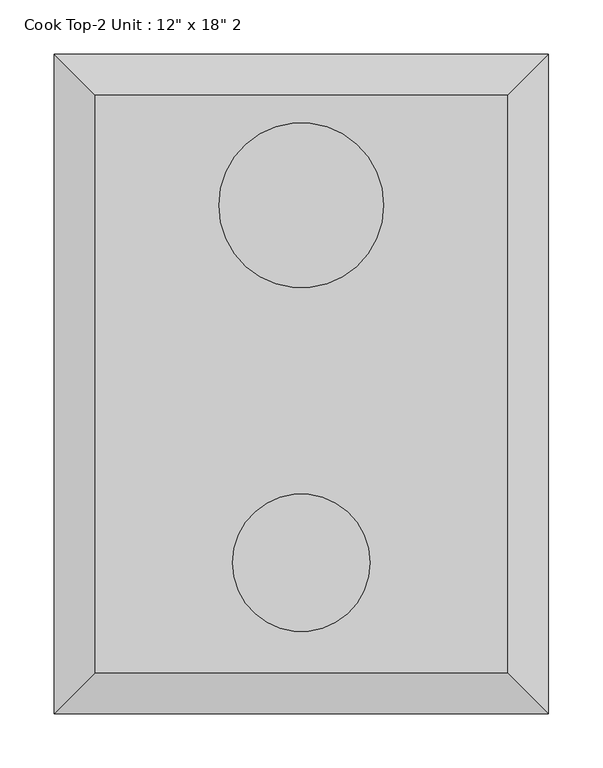
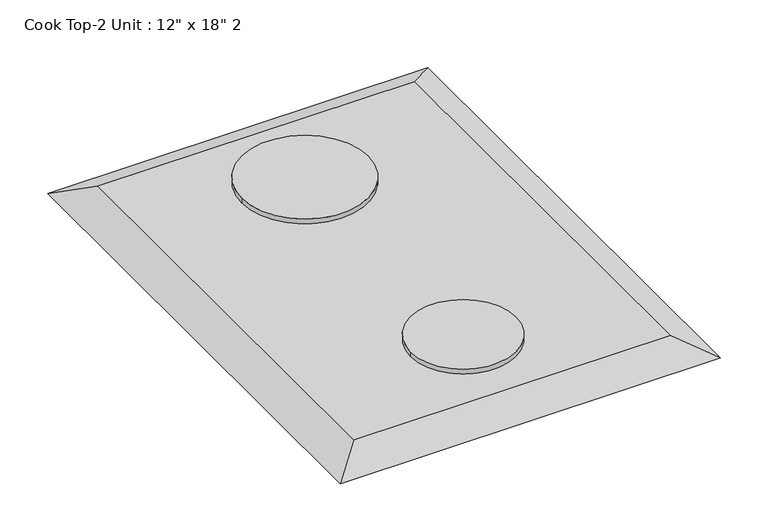
"""IFC4 building model written with IfcOpenShell, lengths in millimetres: proxy geometry."""

from ifc_helpers import new_model, si_unit, point, frame, frame_2d, origin, place, context, project, spatial, circle_curve, trimmed, segment, composite_curve, outline, extrude, faceted_brep, source, transform, mapped, element, save


def proxy_3c1fa1d0(model_context):
    return source(origin(), model_context, "Body", "SolidModel", [
        faceted_brep([(266.7, 296.9247956, 933.45), (-114.3, 296.9247956, 933.45), (-114.3, -236.4752044, 933.45), (266.7, -236.4752044, 933.45), (304.8, 335.0247956, 914.4), (304.8, -274.5752044, 914.4), (-152.4, -274.5752044, 914.4), (-152.4, 335.0247956, 914.4)], [[[0, 1, 2, 3]], [[4, 5, 6, 7]], [[4, 7, 1, 0]], [[7, 6, 2, 1]], [[6, 5, 3, 2]], [[5, 4, 0, 3]]]),
        extrude(outline(composite_curve([segment(trimmed(circle_curve(frame_2d((76.2, 195.3247956)), 76.2), [point((152.4, 195.3247956))], [point((0.0, 195.3247956))], False, "CARTESIAN"), True, "CONTINUOUS"), segment(trimmed(circle_curve(frame_2d((76.2, 195.3247956)), 76.2), [point((0.0, 195.3247956))], [point((152.4, 195.3247956))], False, "CARTESIAN"), True, "CONTINUOUS")], self_intersect=False)), frame((0.0, 0.0, 933.45), z_axis=(0.0, 0.0, 1.0), x_axis=(1.0, 0.0, 0.0)), (0.0, 0.0, 1.0), 6.35),
        extrude(outline(composite_curve([segment(trimmed(circle_curve(frame_2d((76.2, -134.8752044)), 63.5), [point((139.7, -134.8752044))], [point((12.7, -134.8752044))], False, "CARTESIAN"), True, "CONTINUOUS"), segment(trimmed(circle_curve(frame_2d((76.2, -134.8752044)), 63.5), [point((12.7, -134.8752044))], [point((139.7, -134.8752044))], False, "CARTESIAN"), True, "CONTINUOUS")], self_intersect=False)), frame((0.0, 0.0, 933.45), z_axis=(0.0, 0.0, 1.0), x_axis=(1.0, 0.0, 0.0)), (0.0, 0.0, 1.0), 6.35),
    ])


if __name__ == "__main__":
    model = new_model("IFC4")
    model_context = context("Model", 3, world=origin())
    ifc_project = project(units=[si_unit("LENGTHUNIT", "METRE", prefix="MILLI")], contexts=[model_context])
    site = spatial("IfcSite", under=ifc_project)
    building = spatial("IfcBuilding", under=site)
    placement = place(None, origin())
    proxy_shape = proxy_3c1fa1d0(model_context)
    element("IfcBuildingElementProxy", 1, Name="Cook Top-2 Unit : 12\" x 18\" 2", ObjectType="Cook Top-2 Unit : 12\" x 18\" 2", at=placement, inside=building, context=model_context, shape_type="MappedRepresentation", body=[
        mapped(proxy_shape, transform((0.0, 0.0, 0.0), x_axis=(1.0, 0.0, 0.0), y_axis=(0.0, 1.0, 0.0), z_axis=(0.0, 0.0, 1.0))),
    ])
    save(model, "model.ifc")

# Revit data of these elements
# Type "Cook Top-2 Unit : 12\" x 18\" 2"
#   Assembly Code = "E1090400"
#   Counter Height = 3' - 0"
#   Depth = 2' - 0"
#   Width = 1' - 6"
#   Burner Material = Metal - Chrome
#   Cooktop Material = Metal - Steel, Polished
#   Default Elevation = 0
# Element 1 (IfcBuildingElementProxy, "Cook Top-2 Unit : 12\" x 18\" 2")
#   Materials on its faces: "Metal - Steel, Polished", "Metal - Chrome"
# Materials
#   "Metal - Chrome": colour RGB 17 17 17, transparency 0
#   "Metal - Steel, Polished": colour RGB 57 57 57, transparency 0
